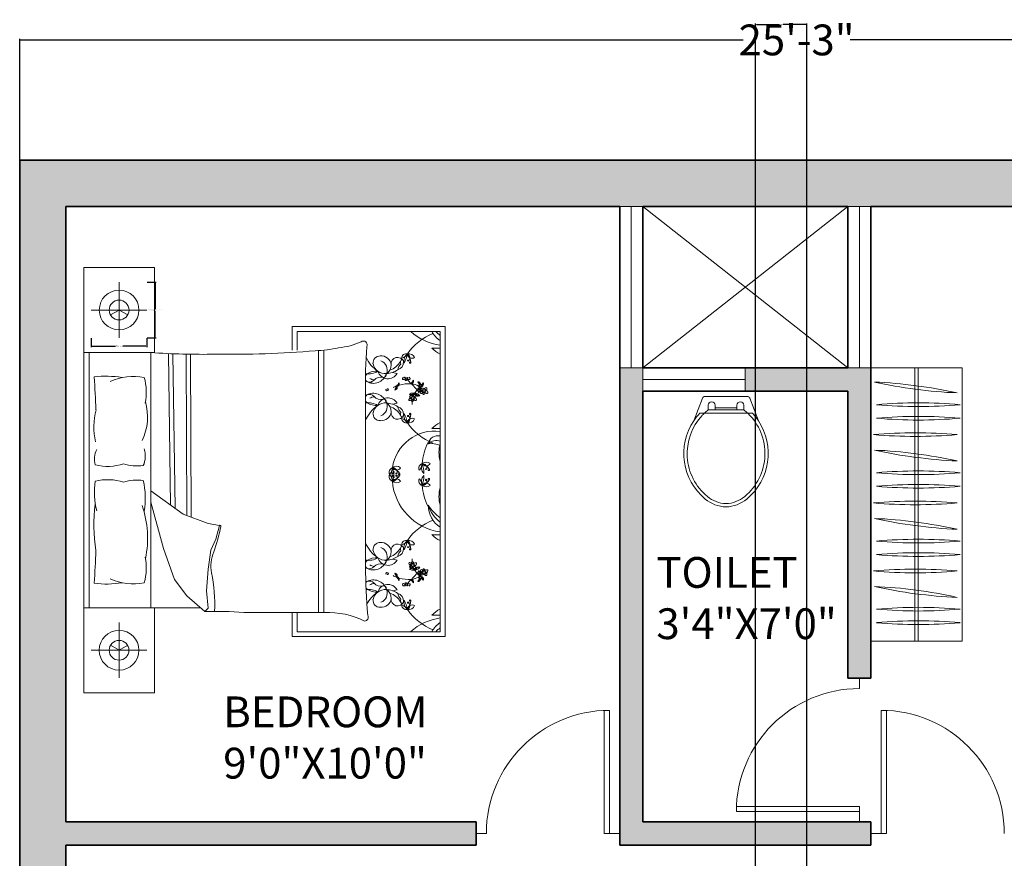
# Model space of a CAD drawing. Units: inches. Extents: x -5 to 366, y -496 to 54.
# Tile 9 of 10: x 22 to 214, y -110 to 54. Entities that reach past the tile are written whole.
import ezdxf

# ---------------------------------------------------------------- set-up
doc = ezdxf.new("R2010")
doc.units = ezdxf.units.IN
doc.header["$MEASUREMENT"] = 0
for name, color, linetype, lineweight in [('A-ANNO-DIMS', 2, 'Continuous', 18), ('A-AREA-IDEN', 7, 'Continuous', 25), ('A-DOOR', 3, 'Continuous', 18), ('A-FLOR-FIXT', 9, 'Continuous', 18), ('A-FLOR-OPEN', 8, 'Continuous', 13), ('A-FURN', 8, 'Continuous', 18), ('A-GLAZ', 4, 'Continuous', 18), ('A-WALL', 7, 'Continuous', 35), ('A-WALL-PATT', 252, 'Continuous', 13)]:
    doc.layers.add(name, color=color, linetype=linetype, lineweight=lineweight)
doc.styles.get("Standard").update_dxf_attribs({"font": 'arial.ttf'})
doc.dimstyles.get("Standard").update_dxf_attribs({"dimtxt": 0.18, "dimasz": 0.18, "dimexe": 0.18, "dimexo": 0.0625, "dimgap": 0.09, "dimtad": 0, "dimtih": 1, "dimtoh": 1, "dimdec": 0, "dimzin": 0, "dimdsep": 46, "dimlunit": 3, "dimtxsty": 'Standard', "dimcen": 0.09, "dimadec": 0, "dimazin": 0, "dimtfac": 1, "dimtdec": 0, "dimtofl": 0, "dimtmove": 0, "dimatfit": 3, "dimfxl": 1, "dimtolj": 1, "dimtzin": 0, "dimarcsym": 0})

# ---------------------------------------------------------------- blocks, each defined once
blk = doc.blocks.new('*D2')
at = {"layer": 'A-ANNO-DIMS', "color": 0, "lineweight": -2, "transparency": 16777216}
for p, q in [((21.93, 26.58), (21.93, 50.16)), ((22.11, 49.98), (162.99, 49.98)), ((324.75, 49.98), (183.88, 49.98)), ((324.93, 26.58), (324.93, 50.16))]:
    blk.add_line(p, q, dxfattribs=at)
at = {"layer": 'A-ANNO-DIMS', "color": 0, "transparency": 16777216}
for points in [[(22.11, 50.01), (22.11, 49.95), (21.93, 49.98)], [(324.75, 50.01), (324.75, 49.95), (324.93, 49.98)]]:
    blk.add_solid(points, dxfattribs=at)
at = {"layer": 'Defpoints', "color": 0, "transparency": 16777216}
for p in [(324.93, 49.98), (21.93, 26.52), (324.93, 26.52)]:
    blk.add_point(p, dxfattribs=at)
at = {"layer": 'A-ANNO-DIMS', "color": 0, "transparency": 16777216, "insert": (173.43, 49.98), "char_height": 6, "attachment_point": 5}
blk.add_mtext('\\A1;25\'-3"', dxfattribs=at)
blk = doc.blocks.new('DOOR-SWING-24IN')
for p, q in [((-1, 0), (-1, 24)), ((0, 0), (0, 24))]:
    blk.add_line(p, q)
blk.add_arc((0, 0), 24, 90, 180)
blk = doc.blocks.new('WARDROBE-HANGING')
for p, q in [((0, 53.26), (0, 0)), ((0, 53.26), (17.76, 53.26)), ((8.58, 53.26), (8.58, 0)), ((9.18, 53.26), (9.18, 0)), ((17.76, 53.26), (17.76, 0)), ((0, 0), (17.76, 0))]:
    blk.add_line(p, q)
for centre, start, end in [((20.87, 141.73), 257.508, 267.5023), ((-3.4, -42.81), 77.508, 87.5023), ((9.24, -46.96), 85.0028, 94.9972), ((9.24, 139.16), 265.0028, 274.9972), ((9.24, -49.59), 85.0028, 94.9972), ((9.24, 136.53), 265.0028, 274.9972), ((8.66, -52.79), 85.0028, 94.9972), ((8.66, 133.34), 265.0028, 274.9972), ((20.87, 128.46), 257.508, 267.5023), ((-3.4, -56.08), 77.508, 87.5023), ((9.24, -60.23), 85.0028, 94.9972), ((9.24, 125.89), 265.0028, 274.9972), ((9.24, -62.86), 85.0028, 94.9972), ((9.24, 123.26), 265.0028, 274.9972), ((8.66, -66.11), 85.0028, 94.9972), ((8.66, 120.02), 265.0028, 274.9972), ((-3.4, -69.4), 77.508, 87.5023), ((20.87, 115.14), 257.508, 267.5023), ((9.24, -73.55), 85.0028, 94.9972), ((9.24, 112.57), 265.0028, 274.9972), ((9.24, -76.18), 85.0028, 94.9972), ((9.24, 109.94), 265.0028, 274.9972), ((8.66, -79.38), 85.0028, 94.9972), ((8.66, 106.75), 265.0028, 274.9972), ((-3.4, -82.67), 77.508, 87.5023), ((20.87, 101.87), 257.508, 267.5023), ((9.24, -86.82), 85.0028, 94.9972), ((9.24, 99.3), 265.0028, 274.9972), ((9.24, -89.45), 85.0028, 94.9972), ((9.24, 96.67), 265.0028, 274.9972)]:
    blk.add_arc(centre, 93.42, start, end)
blk = doc.blocks.new('LAMP-BEDSIDE')
for p, q in [((5.42, 0), (5.42, 10.83)), ((10.83, 5.42), (0, 5.42))]:
    blk.add_line(p, q)
for points in [[(5.42, 5.42), (3.74, 4.45)], [(5.42, 5.42), (7.09, 4.45)]]:
    blk.add_lwpolyline(points)
for radius in [3.87, 1.93]:
    blk.add_circle((5.42, 5.42), radius)
blk = doc.blocks.new('*D23')
at = {"layer": 'A-ANNO-DIMS', "color": 0, "lineweight": -2, "transparency": 16777216}
for p, q in [((46.8, 2.73), (48.54, 2.73)), ((48.36, 2.55), (48.36, -2.5)), ((48.36, -7.92), (48.36, -2.87)), ((46.8, -8.1), (48.54, -8.1))]:
    blk.add_line(p, q, dxfattribs=at)
at = {"layer": 'A-ANNO-DIMS', "color": 0, "transparency": 16777216}
for points in [[(48.33, 2.55), (48.39, 2.55), (48.36, 2.73)], [(48.33, -7.92), (48.39, -7.92), (48.36, -8.1)]]:
    blk.add_solid(points, dxfattribs=at)
at = {"layer": 'Defpoints', "color": 0, "transparency": 16777216}
for p in [(46.73, 2.73), (48.36, 2.73), (46.73, -8.1)]:
    blk.add_point(p, dxfattribs=at)
at = {"layer": 'A-ANNO-DIMS', "color": 0, "transparency": 16777216, "insert": (48.36, -2.68), "char_height": 0.18, "attachment_point": 5}
blk.add_mtext('\\A1;BEDSIDE LAMP 0\'-11" TYP.', dxfattribs=at)
blk = doc.blocks.new('*D24')
at = {"layer": 'A-ANNO-DIMS', "color": 0, "lineweight": -2, "transparency": 16777216}
for p, q in [((35.9, -8.16), (35.9, -9.9)), ((46.73, -8.16), (46.73, -9.9)), ((36.08, -9.72), (40.61, -9.72)), ((46.55, -9.72), (42.02, -9.72))]:
    blk.add_line(p, q, dxfattribs=at)
at = {"layer": 'A-ANNO-DIMS', "color": 0, "transparency": 16777216}
for points in [[(36.08, -9.69), (36.08, -9.75), (35.9, -9.72)], [(46.55, -9.69), (46.55, -9.75), (46.73, -9.72)]]:
    blk.add_solid(points, dxfattribs=at)
at = {"layer": 'Defpoints', "color": 0, "transparency": 16777216}
for p in [(35.9, -8.1), (46.73, -8.1), (46.73, -9.72)]:
    blk.add_point(p, dxfattribs=at)
at = {"layer": 'A-ANNO-DIMS', "color": 0, "transparency": 16777216, "insert": (41.32, -9.72), "char_height": 0.18, "attachment_point": 5}
blk.add_mtext('\\A1;0\'-11" TYP.', dxfattribs=at)
blk = doc.blocks.new('*D29')
at = {"layer": 'A-ANNO-DIMS', "color": 0, "lineweight": -2, "transparency": 16777216}
for p, q in [((165.43, -380.42), (165.43, 53.15)), ((165.61, 52.97), (170.03, 52.97)), ((175.25, 52.97), (170.83, 52.97)), ((175.43, -380.42), (175.43, 53.15))]:
    blk.add_line(p, q, dxfattribs=at)
at = {"layer": 'A-ANNO-DIMS', "color": 0, "transparency": 16777216}
for points in [[(165.61, 53), (165.61, 52.94), (165.43, 52.97)], [(175.25, 53), (175.25, 52.94), (175.43, 52.97)]]:
    blk.add_solid(points, dxfattribs=at)
at = {"layer": 'Defpoints', "color": 0, "transparency": 16777216}
for p in [(175.43, 52.97), (165.43, -380.48), (175.43, -380.48)]:
    blk.add_point(p, dxfattribs=at)
at = {"layer": 'A-ANNO-DIMS', "color": 0, "transparency": 16777216, "insert": (170.43, 52.97), "char_height": 0.18, "attachment_point": 5}
blk.add_mtext('\\A1;0\'-10"', dxfattribs=at)

msp = doc.modelspace()

# ---------------------------------------------------------------- hatches: boundary and pattern name
at = {"layer": 'A-WALL-PATT'}
h = msp.add_hatch(color=256, dxfattribs=at)
h.dxf.hatch_style = 1
h.paths.add_polyline_path([(324.93, 26.52), (21.93, 26.52), (21.93, -456.98), (26.43, -456.98), (26.43, -331.98), (30.93, -331.98), (30.93, -322.98), (30.93, -106.98), (110.93, -106.98), (110.93, -104.73), (110.93, -102.48), (30.93, -102.48), (30.93, 17.52), (138.93, 17.52), (141.18, 17.52), (143.43, 17.52), (183.43, 17.52), (187.93, 17.52), (315.93, 17.52), (315.93, -102.48), (315.93, -106.98), (315.93, -255.48), (171.93, -255.48), (171.93, -155.84), (167.43, -155.84), (167.43, -291.98), (171.93, -291.98), (171.93, -259.98), (315.93, -259.98), (315.93, -375.98), (297.93, -375.98), (297.93, -380.48), (315.93, -380.48), (315.93, -452.48), (315.93, -456.98), (324.93, -456.98)])
h.paths.add_polyline_path([(143.43, -18.48), (143.43, -13.98), (138.93, -13.98), (138.93, -106.98), (187.93, -106.98), (187.93, -102.48), (143.43, -102.48)], flags=17)
h = msp.add_hatch(color=256, dxfattribs=at)
h.dxf.hatch_style = 1
h.paths.add_polyline_path([(187.93, -13.98), (183.43, -13.98), (163.43, -13.98), (163.43, -18.48), (183.43, -18.48), (183.43, -74.48), (185.68, -74.48), (187.93, -74.48)])
h.paths.add_polyline_path([(284.93, -102.48), (215.93, -102.48), (215.93, -104.73), (215.93, -106.98), (280.43, -106.98), (284.93, -106.98)])
h.paths.add_polyline_path([(284.93, -133.23), (280.43, -133.23), (280.43, -154.98), (220.43, -154.98), (220.43, -134.98), (215.93, -134.98), (215.93, -159.48), (284.93, -159.48)])
h.paths.add_polyline_path([(139.43, -322.98), (123.64, -322.98), (123.64, -331.98), (139.43, -331.98)])
h.paths.add_polyline_path([(171.93, -319.98), (167.43, -319.98), (167.43, -331.98), (171.93, -331.98)])
h.paths.add_polyline_path([(269.93, -375.98), (171.93, -375.98), (167.43, -375.98), (167.43, -380.48), (171.93, -380.48), (265.43, -380.48), (265.43, -452.48), (171.93, -452.48), (167.43, -452.48), (167.43, -456.98), (281.67, -456.98), (281.67, -452.48), (269.93, -452.48), (269.93, -380.48)])

# ---------------------------------------------------------------- linework, layer by layer
at = {"layer": 'A-DOOR'}
for p, q in [((185.68, -76.48), (185.68, -74.48)), ((185.68, -102.48), (185.68, -99.48)), ((112.93, -104.73), (110.93, -104.73)), ((138.93, -104.73), (135.93, -104.73)), ((187.93, -104.73), (190.93, -104.73))]:
    msp.add_line(p, q, dxfattribs=at)
at = {"layer": 'A-FLOR-FIXT'}
for p, q in [((154.53, -22.8), (155.43, -22.8)), ((155.43, -22.8), (159.67, -22.8)), ((163.91, -22.8), (159.67, -22.8)), ((163.91, -22.8), (164.81, -22.8))]:
    msp.add_line(p, q, dxfattribs=at)
for points in [[(159.67, -19.54), (155.56, -19.54, 0.31031), (155.05, -19.89), (153.36, -24.28, 0.209071)], [(156.18, -22.15), (156.18, -21.25, -1), (157.55, -21.25), (157.55, -21.72)], [(159.67, -19.54), (163.78, -19.54, -0.31031), (164.29, -19.89), (165.98, -24.28, -0.209071)], [(163.16, -22.15), (163.16, -21.25, 1), (161.79, -21.25), (161.79, -21.72)], [(154.53, -22.8, 0.040937), (153.36, -24.28, 0.163732)], [(155.43, -22.8, 0.014165), (155, -23.24, 0.162618)], [(156.18, -22.15, 0.022712), (155.43, -22.8, 0.162618)], [(159.67, -22.15), (156.18, -22.15, 0.022712)], [(159.67, -22.15), (163.16, -22.15, -0.476108)], [(163.91, -22.8, -0.448546), (163.31, -39.03, -0.162618), (159.67, -40.43, -0.470877)], [(163.16, -22.15, -0.022712), (163.91, -22.8, -0.162618)], [(164.81, -22.8, -0.040937), (165.98, -24.28, -0.163732)], [(153.36, -24.28, 0.383919), (155.62, -39.53, 0.163732), (159.67, -41.08, 0.359733)], [(155, -23.24, 0.431639), (156.03, -39.03, 0.162618), (159.67, -40.43, 0.470877)], [(165.98, -24.28, -0.383919), (163.72, -39.53, -0.163732), (159.67, -41.08, -0.359733)]]:
    msp.add_lwpolyline(points, format="xyb", dxfattribs=at)
for points in [[(161.79, -21.72), (157.55, -21.72)], [(157.55, -21.72), (157.55, -22.15)], [(161.79, -21.72), (161.79, -22.15)]]:
    msp.add_lwpolyline(points, dxfattribs=at)
at = {"layer": 'A-FLOR-OPEN'}
for p, q in [((143.43, 17.52), (183.43, -13.98)), ((183.43, 17.52), (143.43, -13.98))]:
    msp.add_line(p, q, dxfattribs=at)
at = {"layer": 'A-FURN'}
for p, q in [((34.41, -77.29), (34.41, 5.61)), ((75.05, -10.51), (75.05, -5.91)), ((75.05, -5.91), (104.91, -5.91)), ((76.01, -6.87), (76.01, -10.53)), ((103.95, -6.87), (76.01, -6.87)), ((103.95, -65.39), (103.95, -6.87)), ((104.91, -5.91), (104.91, -66.35)), ((35.47, -10.97), (35.47, -60.71)), ((47.51, -60.71), (47.51, -10.97)), ((50.95, -11.2), (51.37, -40.71)), ((51.8, -11.23), (52.23, -41.33)), ((54.41, -11.27), (54.54, -42.75)), ((55.26, -11.27), (55.4, -43.08)), ((80.22, -10.6), (80.22, -61.67)), ((81.25, -10.52), (81.25, -61.67)), ((95.54, -15.04), (94.61, -14.86)), ((89.39, -19.01), (89.39, -52.67)), ((95.54, -20.84), (94.61, -21.02)), ((47.51, -37.94), (53.83, -42.48)), ((49.97, -49.2), (47.51, -40.16)), ((53.83, -42.48), (58.7, -44.33)), ((58.7, -44.33), (60.88, -44.67)), ((60.88, -44.67), (60.21, -47.35)), ((60.21, -47.35), (59.2, -49.53)), ((52.15, -55.24), (49.97, -49.2)), ((59.2, -49.53), (58.7, -53.23)), ((95.54, -51.43), (94.61, -51.25)), ((58.7, -53.23), (58.36, -57.43)), ((54.5, -58.43), (52.15, -55.24)), ((58.36, -57.43), (58.7, -60.78)), ((95.54, -57.22), (94.61, -57.41)), ((58.03, -61.46), (54.5, -58.43)), ((34.41, -60.71), (57.16, -60.71)), ((58.7, -60.78), (58.03, -61.46)), ((75.05, -66.35), (75.05, -61.66)), ((76.01, -61.67), (76.01, -65.39)), ((104.91, -66.35), (75.05, -66.35)), ((76.01, -65.39), (103.95, -65.39))]:
    msp.add_line(p, q, dxfattribs=at)
for points in [[(34.41, -10.97), (48.22, -10.97), (48.22, 5.61), (34.41, 5.61)], [(48.22, -60.71), (48.22, -77.29), (34.41, -77.29)]]:
    msp.add_lwpolyline(points, dxfattribs=at)
for points in [[(79.56, -10.62, 0.056112), (84.13, -10.02, 0.095341), (88.52, -8.85)], [(36.47, -15.73, -0.074897), (41.89, -15.84, 0.472817)], [(42.19, -32.69, -0.14099), (36.67, -32.86, -0.235245)], [(42.19, -36.23, 0.14099), (36.67, -36.07, 0.235245)], [(36.47, -55.95, 0.074897), (41.89, -55.85, -0.472817)], [(65.62, -61.63, 0.001242), (81.35, -61.67, -0.127202), (89.19, -63.33)]]:
    msp.add_lwpolyline(points, format="xyb", dxfattribs=at)
for centre in [(100.77, -18.45), (98.55, -19.83), (98.55, -52.43), (100.77, -53.81)]:
    msp.add_circle(centre, 0.211, dxfattribs=at)
for centre, radius, start, end in [((106.48, -17.34), 10.83, 111.4092, 145.6135), ((105.41, 1.19), 10.83, 228.1144, 262.255), ((106.86, -4.25), 5.28, 209.8884, 236.5383), ((107.84, -2.35), 6.57, 223.5186, 233.6964), ((88.94, -9.48), 0.756, 336.5219, 123.8264), ((57.64, 137.64), 148.96, 266.1, 270.9282), ((63.06, 182.99), 194.31, 269.1145, 274.8735), ((170.02, -16.48), 80.67, 175.2402, 181.8035), ((97.33, -12.09), 0.897, 76.272, 177.0484), ((95.97, -10.26), 1.85, 284.7031, 328.6173), ((98.55, -12.61), 1.71, 125.7657, 194.5347), ((90.15, -9.58), 7.57, 332.8176, 347.4827), ((97.8, -12.39), 1.2, 20.9613, 102.2885), ((98.45, -11.19), 0.904, 181.7131, 301.5367), ((95.48, -13.02), 2.74, 2.0648, 41.1598), ((97.13, -12.01), 0.886, 316.2238, 62.3173), ((105.64, -7.2), 4.4, 221.0454, 247.4453), ((103.27, 4.86), 14.98, 266.3481, 272.5919), ((95.23, -9.37), 6.27, 203.6453, 236.3329), ((92.22, -13.03), 1.4, 88.9462, 185.5144), ((93.26, -12.6), 2.49, 193.079, 274.7067), ((92.42, -13.6), 1.98, 7.1143, 95.0551), ((91.67, -14.38), 1.92, 338.5779, 68.4181), ((91.98, -13.26), 2.41, 305.9599, 357.6409), ((92.87, -10.68), 3.91, 288.2955, 328.7386), ((95.61, -13.15), 1.24, 19.1312, 189.736), ((95.24, -12.85), 1.55, 285.6955, 4.031), ((97.3, -14.52), 1.65, 128.4175, 173.8338), ((96.96, -12.89), 0.763, 126.7319, 206.0245), ((97.64, -12.52), 0.0706, 20.2667, 316.2271), ((98.02, -12.92), 0.0653, 52.0591, 168.5166), ((98.09, -12.93), 0.134, 168.5166, 2.0648), ((90.31, -15.93), 0.998, 127.675, 162.5814), ((90.01, -11.68), 3.43, 259.249, 301.1782), ((90.9, -14.34), 2.64, 240.8249, 340.7178), ((91.5, -17.78), 3.2, 85.2696, 124.215), ((93.76, -14.02), 2.06, 196.8663, 330.0915), ((92.89, -15.32), 0.515, 254.8529, 12.6959), ((91.5, -17.78), 3.2, 53.6555, 57.2989), ((93.19, -10.64), 4.45, 273.4924, 303.7117), ((-752.48, -61.43), 790.27, 2.85022, 3.31479), ((44.06, -26.3), 10.68, 78.2417, 114.8684), ((35.5, -18.69), 11.11, 348.9631, 14.8961), ((90.31, -15.93), 0.998, 196.6343, 225.5483), ((90.11, -15.51), 1.24, 246.1646, 318.4347), ((91.38, -13.94), 2.38, 240.0851, 262.564), ((92.31, -17.46), 1.7, 74.8529, 138.4347), ((95.54, -17.17), 0.398, 265.7131, 351.6568), ((94.67, -16.35), 1.33, 313.6929, 321.7899), ((96.14, -17.26), 0.435, 115.5379, 168.6744), ((94.67, -16.64), 1.31, 329.344, 349.7412), ((97.85, -23.93), 6.87, 86.1723, 106.4158), ((93.62, -16.94), 2.34, 352.8698, 1.6736), ((96.72, -16.1), 0.163, 125.0752, 284.7644), ((96.97, -16.03), 0.352, 127.3642, 168.4363), ((96.69, -15.75), 0.508, 277.4968, 341.2737), ((97.09, -15.99), 0.202, 88.1325, 178.8919), ((97.5, -16.2), 0.436, 136.3462, 189.6513), ((97.25, -16.24), 0.182, 189.6513, 312.3208), ((97.29, -15.74), 0.211, 183.2768, 356.7232), ((97.95, -16.12), 0.691, 164.2829, 186.9148), ((97.14, -16.12), 0.345, 312.3208, 40.2111), ((97.87, -15.73), 0.491, 201.6382, 274.947), ((97.22, -16.4), 0.641, 42.3896, 66.5724), ((103.69, -11.33), 7.87, 217.9541, 226.8459), ((97.68, -16.03), 0.349, 10.9597, 52.2379), ((97.9, -16.06), 0.162, 274.947, 37.5263), ((98.44, -16.98), 0.169, 112.5583, 214.2343), ((98.33, -16.68), 0.398, 265.7131, 351.6568), ((97.98, -16.46), 0.695, 297.3659, 329.344), ((98.02, -20.5), 3.44, 60.7959, 85.244), ((90.69, -25.46), 11.33, 37.8256, 47.7588), ((97.46, -15.86), 1.33, 313.6929, 321.7899), ((98.93, -16.77), 0.435, 115.5379, 168.6744), ((97.45, -16.14), 1.31, 329.344, 349.7412), ((96.41, -16.44), 2.34, 352.8698, 1.6736), ((99.7, -16.92), 0.236, 33.0979, 123.1364), ((94.5, -20.24), 6.17, 31.1156, 34.8118), ((99.35, -17.32), 0.638, 2.3172, 70.5201), ((99.57, -17.18), 0.244, 315.7354, 31.1156), ((99.59, -17.25), 0.55, 352.6008, 57.1845), ((100.12, -17.13), 0.55, 252.8042, 349.6943), ((100.18, -17.08), 0.244, 248.2452, 323.6254), ((99.96, -16.93), 0.638, 291.7087, 3.0299), ((95.41, -13.57), 6.17, 323.6254, 327.3216), ((100.47, -17.09), 0.236, 325.6077, 55.6462), ((90.9, -21.55), 2.64, 19.2822, 119.1751), ((90.11, -20.37), 1.24, 41.5653, 113.8354), ((93.57, -18.16), 0.26, 169.5864, 349.5616), ((93.67, -18.18), 0.16, 349.5616, 167.2949), ((97.85, -23.93), 6.87, 110.1059, 116.9968), ((95.54, -18.27), 0.435, 129.5056, 182.6421), ((94.29, -17.26), 1.31, 308.4388, 328.836), ((94.06, -16.19), 2.34, 296.5064, 305.3102), ((94.04, -17.4), 1.33, 336.3901, 344.4871), ((95.5, -17.74), 0.169, 83.9457, 185.6216), ((94.82, -17.58), 0.695, 328.836, 0.8141), ((95.18, -17.78), 0.398, 306.5232, 32.4668), ((95.65, -17.47), 0.169, 112.5583, 214.2343), ((95.19, -16.95), 0.695, 297.3659, 329.344), ((98.23, -18.22), 0.962, 253.6301, 325.4631), ((98.51, -19.55), 0.681, 82.0748, 142.6895), ((98.43, -18.62), 0.699, 228.342, 274.9894), ((98.45, -18.73), 0.585, 273.8774, 357.1501), ((98.68, -18.32), 0.566, 262.0748, 308.2393), ((102.59, -20.86), 4.13, 156.1523, 156.9499), ((98.95, -19.39), 0.209, 44.3732, 121.9501), ((99.59, -18.9), 0.585, 181.4625, 249.4747), ((102.59, -20.86), 4.13, 130.182, 149.456), ((99.49, -18.44), 0.566, 215.1128, 261.2773), ((99.94, -18.47), 0.962, 197.889, 269.722), ((99.3, -19.67), 0.681, 20.6625, 81.2773), ((100.32, -18.51), 0.681, 139.3812, 199.9959), ((99.05, -18.01), 0.962, 310.9365, 22.7695), ((99.49, -18.07), 0.699, 285.6484, 332.2957), ((99.88, -17.48), 0.184, 135.7354, 318.1297), ((99.37, -17.69), 0.566, 319.3812, 5.5456), ((100.02, -17.48), 0.184, 68.2452, 250.6395), ((101.56, -20.94), 3.68, 111.7087, 116.2181), ((98.02, -20.5), 3.44, 47.5083, 55.9967), ((99.59, -18.11), 0.585, 331.1838, 51.6792), ((100.2, -18.81), 0.163, 125.0752, 284.7644), ((100.45, -18.74), 0.352, 93.635, 168.4363), ((100.4, -18.19), 0.207, 138.2946, 276.2474), ((100.17, -18.46), 0.508, 277.4968, 341.2737), ((100.48, -18.22), 0.288, 358.5719, 143.8954), ((100.57, -18.7), 0.202, 88.1325, 178.8919), ((100.65, -17.99), 0.291, 208.8493, 269.9355), ((100.4, -18.06), 0.332, 274.2123, 318.1587), ((100.98, -18.91), 0.436, 136.3462, 189.6513), ((100.73, -18.96), 0.182, 189.6513, 312.3208), ((101.43, -18.83), 0.691, 164.2829, 186.9148), ((101.41, -18.4), 0.666, 121.9501, 165.2442), ((100.62, -18.83), 0.345, 312.3208, 40.2111), ((101.35, -18.45), 0.491, 201.6382, 274.947), ((100.95, -18.14), 0.14, 262.868, 7.094), ((100.7, -19.12), 0.641, 42.3896, 66.5724), ((100.94, -18.02), 0.417, 278.5614, 22.5914), ((101.17, -18.74), 0.349, 10.9597, 118.7804), ((101.17, -18.01), 0.209, 44.3732, 121.9501), ((101.38, -18.77), 0.162, 274.947, 37.5263), ((36.32, -23.49), 10.55, 333.8761, 16.1746), ((90.31, -19.95), 0.998, 134.4517, 156.7144), ((90.31, -19.95), 0.998, 203.2856, 232.325), ((90.01, -24.21), 3.43, 58.8218, 100.2867), ((91.5, -18.1), 3.2, 235.785, 274.7304), ((91.38, -21.94), 2.38, 97.436, 119.9149), ((93.26, -23.28), 2.49, 85.2933, 166.921), ((92.31, -18.42), 1.7, 221.5653, 285.1471), ((93.76, -21.87), 2.06, 29.9085, 163.1337), ((91.67, -21.5), 1.92, 291.5819, 21.4221), ((92.89, -20.56), 0.515, 347.3041, 105.1471), ((91.5, -18.1), 3.2, 302.7011, 306.3445), ((91.98, -22.62), 2.41, 2.3591, 54.0401), ((93.19, -25.24), 4.45, 56.2883, 86.5076), ((97.97, -20.19), 0.163, 125.0752, 284.7644), ((98.22, -20.13), 0.352, 93.635, 168.4363), ((98.18, -19.57), 0.207, 138.2946, 276.2474), ((97.95, -19.84), 0.508, 277.4968, 341.2737), ((98.26, -19.6), 0.288, 358.5719, 143.8954), ((98.35, -20.08), 0.202, 88.1325, 178.8919), ((98.42, -19.37), 0.291, 208.8493, 269.9355), ((98.18, -19.44), 0.332, 274.2123, 318.1587), ((98.75, -20.29), 0.436, 136.3462, 189.6513), ((98.5, -20.34), 0.182, 189.6513, 312.3208), ((102.59, -20.86), 4.13, 175.2415, 182.8929), ((99.21, -20.21), 0.691, 164.2829, 186.9148), ((99.19, -19.78), 0.666, 121.9501, 165.2442), ((98.39, -20.22), 0.345, 312.3208, 40.2111), ((99.13, -19.83), 0.491, 201.6382, 274.947), ((98.73, -19.52), 0.14, 262.868, 7.094), ((98.48, -20.5), 0.641, 42.3896, 66.5724), ((98.71, -19.4), 0.417, 278.5614, 22.5914), ((98.94, -20.12), 0.349, 10.9597, 118.7804), ((99.15, -20.15), 0.162, 274.947, 37.5263), ((99.64, -18.8), 0.699, 248.3627, 295.0101), ((50.98, -25.57), 14.57, 166.3427, 191.1841), ((95.23, -26.51), 6.27, 123.6671, 158.5059), ((92.22, -22.85), 1.4, 174.4856, 271.0538), ((92.42, -22.28), 1.98, 264.9449, 352.8857), ((92.87, -25.2), 3.91, 31.2614, 71.7045), ((95.61, -22.73), 1.24, 170.264, 340.8688), ((97.3, -21.36), 1.65, 186.1662, 231.5825), ((95.24, -23.03), 1.55, 355.969, 74.3045), ((96.96, -22.99), 0.763, 153.9755, 233.2681), ((98.55, -23.27), 1.71, 165.4653, 234.2343), ((90.15, -26.3), 7.57, 12.5173, 27.1824), ((95.48, -22.86), 2.74, 318.8402, 357.9352), ((98.09, -22.95), 0.134, 357.9352, 191.4834), ((98.02, -22.97), 0.0653, 191.4834, 307.9409), ((97.33, -23.79), 0.897, 182.9516, 283.728), ((95.97, -25.62), 1.85, 31.3827, 75.2969), ((97.13, -23.88), 0.886, 297.6827, 43.7762), ((98.45, -24.69), 0.904, 58.4633, 178.2869), ((97.8, -23.49), 1.2, 257.7115, 339.0387), ((106.48, -18.55), 10.83, 214.3865, 248.5908), ((97.69, -23.34), 0.117, 43.7762, 339.7183), ((105.64, -28.68), 4.4, 112.5547, 138.9546), ((102.91, -34.65), 8.38, 82.8636, 171.8197), ((103.27, -40.74), 14.98, 87.4081, 93.6519), ((111.21, -33.47), 10.83, 152.5854, 175.5377), ((103.49, -29.12), 1.94, 76.3898, 169.0739), ((103.23, -30.58), 2.46, 72.8609, 131.9049), ((102.14, -33.57), 4.85, 68.117, 96.6195), ((109.64, -30.45), 5.95, 162.9798, 196.4569), ((40.61, -31.72), 4.1, 153.3437, 196.1026), ((42.04, -31.17), 4.39, 335.0183, 18.5407), ((100.66, -33.49), 0.897, 106.1963, 206.9726), ((98.57, -32.59), 1.85, 314.6273, 358.5415), ((101.97, -33.34), 1.71, 155.6899, 224.4589), ((101.22, -33.52), 1.2, 50.8855, 132.2127), ((101.18, -32.16), 0.904, 211.6373, 331.4609), ((99.53, -35.22), 2.74, 31.989, 71.0841), ((93.19, -34.9), 7.57, 2.7418, 17.407), ((100.45, -33.52), 0.886, 346.148, 92.2415), ((112.71, -32.81), 8.8, 174.3643, 175.6213), ((118.74, -37.44), 15.73, 160.0972, 160.2783), ((44.96, -22.92), 10.16, 254.1707, 275.9871), ((94.87, -34.32), 0.897, 106.1963, 206.9726), ((92.77, -33.41), 1.85, 314.6273, 358.5415), ((96.18, -34.17), 1.71, 155.6899, 224.4589), ((96.18, -35.34), 1.71, 135.5411, 204.3101), ((95.42, -34.35), 1.2, 50.8855, 132.2127), ((95.39, -32.99), 0.904, 211.6373, 331.4609), ((94.65, -34.35), 0.886, 346.148, 92.2415), ((93.73, -36.05), 2.74, 31.989, 71.0841), ((87.39, -35.73), 7.57, 2.7418, 17.407), ((87.39, -33.78), 7.57, 342.593, 357.2582), ((95.35, -34.54), 0.0706, 50.1909, 346.0209), ((101.15, -33.71), 0.0706, 50.1909, 346.0209), ((101.67, -33.87), 0.0653, 81.9833, 198.4408), ((101.73, -33.84), 0.134, 198.4408, 31.989), ((51.28, -38.24), 14.77, 171.5249, 193.96), ((44.96, -46), 10.16, 84.0129, 105.8293), ((31.81, -39.35), 14.62, 349.8617, 13.6238), ((94.87, -35.18), 0.897, 153.0274, 253.8037), ((92.77, -36.09), 1.85, 1.4585, 45.3727), ((93.73, -33.45), 2.74, 288.9159, 328.011), ((94.65, -35.16), 0.886, 267.7585, 13.852), ((95.39, -36.52), 0.904, 28.5391, 148.3627), ((95.42, -35.15), 1.2, 227.7873, 309.1145), ((105.41, -35.2), 10.83, 184.4623, 262.255), ((95.4, -34.97), 0.117, 13.852, 309.9245), ((95.94, -34.67), 0.134, 198.4408, 31.989), ((95.87, -34.69), 0.0653, 81.9833, 198.4408), ((95.94, -34.83), 0.134, 328.011, 161.5592), ((95.87, -34.81), 0.0653, 161.5592, 278.0167), ((100.66, -36.01), 0.897, 153.0274, 253.8037), ((98.57, -36.92), 1.85, 1.4585, 45.3727), ((101.97, -36.17), 1.71, 135.5411, 204.3101), ((93.19, -34.6), 7.57, 342.593, 357.2582), ((99.53, -34.28), 2.74, 288.9159, 328.011), ((100.45, -35.99), 0.886, 267.7585, 13.852), ((101.18, -37.34), 0.904, 28.5391, 148.3627), ((101.19, -35.8), 0.117, 13.852, 309.9245), ((101.67, -35.64), 0.0653, 161.5592, 278.0167), ((101.73, -35.66), 0.134, 328.011, 161.5592), ((101.22, -35.98), 1.2, 227.7873, 309.1145), ((111.21, -36.03), 10.83, 184.4623, 207.4146), ((109.64, -39.06), 5.95, 163.5431, 197.0202), ((112.71, -36.7), 8.8, 184.3787, 185.6357), ((118.74, -32.06), 15.73, 199.7217, 199.9028), ((66.47, -44.59), 30.07, 172.2196, 189.497), ((27.61, -47.15), 19.27, 348.0397, 19.2615), ((106.86, -40.63), 5.28, 181.272, 236.5383), ((109.69, -35.28), 9.78, 214.0123, 234.053), ((107.84, -38.73), 6.57, 197.8504, 233.6964), ((106.48, -53.72), 10.83, 111.4092, 145.6135), ((29.55, -38.91), 32.15, 340.1194, 349.3383), ((60.95, -44.85), 0.2, 358.8623, 109.7536), ((97.33, -48.48), 0.897, 76.272, 177.0484), ((95.97, -46.64), 1.85, 284.7031, 328.6173), ((98.55, -49), 1.71, 125.7657, 194.5347), ((90.15, -45.97), 7.57, 332.8176, 347.4827), ((97.8, -48.78), 1.2, 20.9613, 102.2885), ((97.13, -48.39), 0.886, 316.2238, 62.3173), ((95.48, -49.41), 2.74, 2.0648, 41.1598), ((98.45, -47.58), 0.904, 181.7131, 301.5367), ((103.27, -31.53), 14.98, 266.3481, 272.5919), ((105.64, -43.58), 4.4, 221.0454, 247.4453), ((-752.48, -10.26), 790.27, 356.68521, 357.14978), ((65.96, -52.56), 6.75, 156.2616, 191.3392), ((95.23, -45.76), 6.27, 201.4941, 236.3329), ((92.22, -49.41), 1.4, 88.9462, 185.5144), ((93.26, -48.98), 2.49, 193.079, 274.7067), ((92.42, -49.99), 1.98, 7.1143, 95.0551), ((91.67, -50.77), 1.92, 338.5779, 68.4181), ((91.98, -49.64), 2.41, 305.9599, 357.6409), ((92.87, -47.07), 3.91, 288.2955, 328.7386), ((95.61, -49.53), 1.24, 19.1312, 189.736), ((95.24, -49.23), 1.55, 285.6955, 4.031), ((97.3, -50.91), 1.65, 128.4175, 173.8338), ((96.96, -49.28), 0.763, 126.7319, 206.0245), ((97.64, -48.91), 0.0706, 20.2667, 316.2271), ((98.02, -49.3), 0.0653, 52.0591, 168.5166), ((98.09, -49.31), 0.134, 168.5166, 2.0648), ((35.5, -53), 11.11, 345.1039, 11.0369), ((90.01, -48.06), 3.43, 259.7133, 301.1782), ((90.31, -52.31), 0.998, 127.675, 156.7144), ((90.9, -50.72), 2.64, 240.8249, 340.7178), ((91.5, -54.17), 3.2, 85.2696, 124.215), ((93.76, -50.4), 2.06, 196.8663, 330.0915), ((92.89, -51.71), 0.515, 254.8529, 12.6959), ((91.5, -54.17), 3.2, 53.6555, 57.2989), ((93.19, -47.03), 4.45, 273.4924, 303.7117), ((98.5, -51.93), 0.182, 47.6792, 170.3487), ((102.59, -51.41), 4.13, 177.1071, 184.7585), ((98.39, -52.05), 0.345, 319.7889, 47.6792), ((175.69, -53.66), 86.3, 179.3433, 185.6887), ((90.31, -52.31), 0.998, 203.229, 225.5483), ((90.11, -51.89), 1.24, 246.1646, 318.4347), ((91.38, -50.32), 2.38, 240.0851, 262.564), ((92.31, -53.84), 1.7, 74.8529, 138.4347), ((97.97, -52.08), 0.163, 75.2356, 234.9248), ((98.22, -52.14), 0.352, 191.5637, 266.365), ((98.43, -53.65), 0.699, 85.0106, 131.658), ((98.23, -54.05), 0.962, 34.5369, 106.3699), ((98.51, -52.71), 0.681, 217.3105, 277.9252), ((98.18, -52.7), 0.207, 83.7526, 221.7054), ((97.95, -52.42), 0.508, 18.7263, 82.5032), ((98.26, -52.67), 0.288, 216.1046, 1.4281), ((98.35, -52.19), 0.202, 181.1081, 271.8675), ((98.42, -52.89), 0.291, 90.0645, 151.1507), ((98.18, -52.82), 0.332, 41.8413, 85.7877), ((90.69, -46.81), 11.33, 312.2412, 322.1744), ((98.75, -51.97), 0.436, 170.3487, 223.6538), ((98.45, -53.54), 0.585, 2.8499, 86.1226), ((99.21, -52.06), 0.691, 173.0852, 195.7171), ((99.19, -52.49), 0.666, 194.7558, 238.0499), ((98.68, -53.95), 0.566, 51.7607, 97.9252), ((99.13, -52.44), 0.491, 85.053, 158.3618), ((98.73, -52.75), 0.14, 352.906, 97.132), ((98.48, -51.77), 0.641, 293.4276, 317.6104), ((98.94, -52.15), 0.349, 241.2196, 349.0403), ((98.71, -52.86), 0.417, 337.4086, 81.4386), ((102.59, -51.41), 4.13, 203.0501, 203.8477), ((98.95, -52.88), 0.209, 238.0499, 315.6268), ((99.59, -53.37), 0.585, 110.5253, 178.5375), ((99.94, -53.8), 0.962, 90.278, 162.111), ((99.49, -53.83), 0.566, 98.7227, 144.8872), ((102.59, -51.41), 4.13, 210.544, 229.818), ((99.15, -52.11), 0.162, 322.4737, 85.053), ((99.64, -53.47), 0.699, 64.9899, 111.6373), ((99.3, -52.6), 0.681, 278.7227, 339.3375), ((100.32, -53.76), 0.681, 160.0041, 220.6188), ((99.05, -54.25), 0.962, 337.2305, 49.0635), ((99.49, -54.2), 0.699, 27.7043, 74.3516), ((100.2, -53.46), 0.163, 75.2356, 234.9248), ((100.45, -53.52), 0.352, 191.5637, 266.365), ((100.17, -53.8), 0.508, 18.7263, 82.5032), ((100.57, -53.57), 0.202, 181.1081, 271.8675), ((100.98, -53.35), 0.436, 170.3487, 223.6538), ((100.73, -53.31), 0.182, 47.6792, 170.3487), ((101.43, -53.44), 0.691, 173.0852, 195.7171), ((100.62, -53.43), 0.345, 319.7889, 47.6792), ((101.35, -53.82), 0.491, 85.053, 158.3618), ((100.7, -53.15), 0.641, 293.4276, 317.6104), ((101.17, -53.53), 0.349, 241.2196, 349.0403), ((101.38, -53.49), 0.162, 322.4737, 85.053), ((44.06, -45.39), 10.68, 245.1316, 281.7583), ((28.67, -60.04), 31.29, 357.4519, 11.3392), ((90.31, -56.34), 0.998, 134.4517, 153.558), ((90.9, -57.93), 2.64, 19.2822, 119.1751), ((90.11, -56.76), 1.24, 41.5653, 113.8354), ((93.57, -54.11), 0.26, 10.4384, 190.4136), ((93.67, -54.09), 0.16, 192.7051, 10.4384), ((97.85, -48.34), 6.87, 243.0032, 249.8941), ((94.29, -55.01), 1.31, 31.164, 51.5612), ((95.54, -54), 0.435, 177.3579, 230.4944), ((94.06, -56.07), 2.34, 54.6898, 63.4936), ((94.04, -54.87), 1.33, 15.5129, 23.6099), ((95.5, -54.53), 0.169, 174.3784, 276.0543), ((94.82, -54.69), 0.695, 359.1859, 31.164), ((95.18, -54.48), 0.398, 327.5332, 53.4768), ((95.65, -54.79), 0.169, 145.7657, 247.4417), ((95.54, -55.1), 0.398, 8.3432, 94.2869), ((95.19, -55.32), 0.695, 30.656, 62.6341), ((94.67, -55.91), 1.33, 38.2101, 46.3071), ((96.14, -55), 0.435, 191.3256, 244.4621), ((94.67, -55.63), 1.31, 10.2588, 30.656), ((97.85, -48.34), 6.87, 253.5842, 273.8277), ((93.62, -55.33), 2.34, 358.3264, 7.1302), ((103.69, -60.93), 7.87, 133.1541, 142.0459), ((98.44, -55.29), 0.169, 145.7657, 247.4417), ((98.02, -51.76), 3.44, 274.756, 299.2041), ((98.33, -55.59), 0.398, 8.3432, 94.2869), ((97.98, -55.81), 0.695, 30.656, 62.6341), ((97.46, -56.41), 1.33, 38.2101, 46.3071), ((98.93, -55.5), 0.435, 191.3256, 244.4621), ((97.45, -56.12), 1.31, 10.2588, 30.656), ((96.41, -55.82), 2.34, 358.3264, 7.1302), ((99.35, -54.95), 0.638, 289.4799, 357.6828), ((94.5, -52.03), 6.17, 325.1882, 328.8844), ((99.7, -55.35), 0.236, 236.8636, 326.9021), ((99.88, -54.79), 0.184, 41.8703, 224.2646), ((99.57, -55.09), 0.244, 328.8844, 44.2646), ((99.37, -54.57), 0.566, 354.4544, 40.6188), ((100.02, -54.79), 0.184, 109.3605, 291.7548), ((99.59, -55.02), 0.55, 302.8155, 7.3992), ((101.56, -51.33), 3.68, 243.7819, 248.2913), ((98.02, -51.76), 3.44, 304.0033, 312.4917), ((99.59, -54.16), 0.585, 308.3208, 28.8162), ((100.12, -55.14), 0.55, 10.3057, 107.1958), ((100.18, -55.19), 0.244, 36.3746, 111.7548), ((100.4, -54.08), 0.207, 83.7526, 221.7054), ((99.96, -55.34), 0.638, 356.9701, 68.2913), ((100.48, -54.05), 0.288, 216.1046, 1.4281), ((95.41, -58.7), 6.17, 32.6784, 36.3746), ((100.65, -54.27), 0.291, 90.0645, 151.1507), ((100.4, -54.2), 0.332, 41.8413, 85.7877), ((100.47, -55.18), 0.236, 304.3538, 34.3923), ((101.41, -53.87), 0.666, 194.7558, 238.0499), ((100.95, -54.13), 0.14, 352.906, 97.132), ((100.94, -54.24), 0.417, 337.4086, 81.4386), ((101.17, -54.26), 0.209, 238.0499, 315.6268), ((90.31, -56.34), 0.998, 210.0293, 232.325), ((90.01, -60.59), 3.43, 58.8218, 99.1554), ((91.5, -54.48), 3.2, 235.785, 274.7304), ((91.38, -58.33), 2.38, 97.436, 119.9149), ((93.26, -59.67), 2.49, 85.2933, 166.921), ((92.31, -54.81), 1.7, 221.5653, 285.1471), ((93.76, -58.25), 2.06, 29.9085, 163.1337), ((91.67, -57.88), 1.92, 291.5819, 21.4221), ((92.89, -56.95), 0.515, 347.3041, 105.1471), ((91.5, -54.48), 3.2, 302.7011, 306.3445), ((91.98, -59.01), 2.41, 2.3591, 54.0401), ((93.19, -61.62), 4.45, 56.2883, 86.5076), ((96.72, -56.17), 0.163, 75.2356, 234.9248), ((96.97, -56.23), 0.352, 191.5637, 232.6358), ((96.69, -56.52), 0.508, 18.7263, 82.5032), ((97.09, -56.28), 0.202, 181.1081, 271.8675), ((97.5, -56.07), 0.436, 170.3487, 223.6538), ((97.25, -56.02), 0.182, 47.6792, 170.3487), ((97.29, -56.53), 0.211, 3.2768, 176.7232), ((97.95, -56.15), 0.691, 173.0852, 195.7171), ((97.14, -56.14), 0.345, 319.7889, 47.6792), ((97.87, -56.53), 0.491, 85.053, 158.3618), ((97.22, -55.86), 0.641, 293.4276, 317.6104), ((97.68, -56.24), 0.349, 307.7621, 349.0403), ((97.9, -56.21), 0.162, 322.4737, 85.053), ((95.23, -62.89), 6.27, 123.6671, 153.2997), ((92.22, -59.24), 1.4, 174.4856, 271.0538), ((92.42, -58.66), 1.98, 264.9449, 352.8857), ((92.87, -61.59), 3.91, 31.2614, 71.7045), ((95.61, -59.12), 1.24, 170.264, 340.8688), ((95.24, -59.42), 1.55, 355.969, 74.3045), ((97.3, -57.74), 1.65, 186.1662, 231.5825), ((96.96, -59.37), 0.763, 153.9755, 233.2681), ((98.55, -59.66), 1.71, 165.4653, 234.2343), ((90.15, -62.69), 7.57, 12.5173, 27.1824), ((95.48, -59.24), 2.74, 318.8402, 357.9352), ((98.09, -59.34), 0.134, 357.9352, 191.4834), ((98.02, -59.35), 0.0653, 191.4834, 307.9409), ((60.09, -137.47), 76.04, 85.8294, 91.553), ((95.97, -62.01), 1.85, 31.3827, 75.2969), ((97.33, -60.17), 0.897, 182.9516, 283.728), ((97.13, -60.26), 0.886, 297.6827, 43.7762), ((98.45, -61.07), 0.904, 58.4633, 178.2869), ((97.8, -59.87), 1.2, 257.7115, 339.0387), ((106.48, -54.93), 10.83, 214.3865, 248.5908), ((97.69, -59.73), 0.117, 43.7762, 339.7183), ((105.64, -65.07), 4.4, 112.5547, 138.9546), ((89.13, -62.57), 0.765, 273.98, 27.3412), ((105.41, -73.45), 10.83, 97.745, 131.8856), ((103.27, -77.12), 14.98, 87.4081, 93.6519), ((106.86, -68.02), 5.28, 123.4617, 150.1116), ((107.84, -69.92), 6.57, 126.3036, 136.4814)]:
    msp.add_arc(centre, radius, start, end, dxfattribs=at)
at = {"layer": 'A-GLAZ'}
for p, q in [((141.18, 17.52), (138.93, 17.52)), ((141.18, -13.98), (141.18, 17.52)), ((141.18, 17.52), (143.43, 17.52)), ((183.43, 17.52), (187.93, 17.52)), ((185.68, -13.98), (185.68, 17.52)), ((143.43, -13.98), (138.93, -13.98)), ((143.43, -13.98), (143.43, -18.48)), ((163.43, -13.98), (163.43, -18.48)), ((183.43, -13.98), (187.93, -13.98)), ((163.43, -16.23), (143.43, -16.23))]:
    msp.add_line(p, q, dxfattribs=at)
at = {"layer": 'A-WALL'}
for p, q in [((21.93, 26.52), (21.93, -456.98)), ((21.93, 26.52), (324.93, 26.52)), ((30.93, 17.52), (138.93, 17.52)), ((30.93, 17.52), (30.93, -102.48)), ((138.93, 17.52), (138.93, -106.98)), ((143.43, 17.52), (143.43, -13.98)), ((143.43, 17.52), (183.43, 17.52)), ((183.43, 17.52), (183.43, -13.98)), ((187.93, 17.52), (187.93, -74.48)), ((187.93, 17.52), (315.93, 17.52)), ((143.43, -13.98), (183.43, -13.98)), ((143.43, -18.48), (183.43, -18.48)), ((143.43, -18.48), (143.43, -102.48)), ((183.43, -18.48), (183.43, -74.48)), ((185.68, -74.48), (183.43, -74.48)), ((185.68, -74.48), (187.93, -74.48)), ((30.93, -102.48), (110.93, -102.48)), ((110.93, -104.73), (110.93, -102.48)), ((143.43, -102.48), (187.93, -102.48)), ((187.93, -102.48), (187.93, -106.98)), ((110.93, -104.73), (110.93, -106.98)), ((30.93, -106.98), (110.93, -106.98)), ((30.93, -106.98), (30.93, -322.98)), ((138.93, -106.98), (187.93, -106.98))]:
    msp.add_line(p, q, dxfattribs=at)

# ---------------------------------------------------------------- block references
at = {"layer": 'A-DOOR', "extrusion": (0, 0, -1), "zscale": -1, "rotation": 270.0000000000001}
msp.add_blockref('DOOR-SWING-24IN', (-185.68, -100.48), dxfattribs=at)
at = {"layer": 'A-DOOR'}
msp.add_blockref('DOOR-SWING-24IN', (136.93, -104.73), dxfattribs=at)
at = {"layer": 'A-DOOR', "extrusion": (0, 0, -1), "zscale": -1}
msp.add_blockref('DOOR-SWING-24IN', (-189.93, -104.73), dxfattribs=at)
at = {"layer": 'A-FURN'}
for name, p in [('LAMP-BEDSIDE', (35.9, -8.1)), ('WARDROBE-HANGING', (187.93, -67.24))]:
    msp.add_blockref(name, p, dxfattribs=at)
at = {"layer": 'A-FURN', "rotation": 180}
msp.add_blockref('LAMP-BEDSIDE', (46.73, -63.59), dxfattribs=at)

# ---------------------------------------------------------------- texts
at = {"layer": 'A-AREA-IDEN', "char_height": 6, "attachment_point": 1}
for s, insert in [('TOILET\\P3\'4"X7\'0"', (146.09, -50.84)), ('BEDROOM\\P9\'0"X10\'0"', (61.62, -78.02))]:
    msp.add_mtext(s, dxfattribs=dict(at, insert=insert))

# ---------------------------------------------------------------- dimensions: what is measured, and where the dimension line sits
at = {"layer": 'A-ANNO-DIMS'}
for base, p1, p2, override, picture, middle in [((324.93, 49.98), (21.93, 26.52), (324.93, 26.52), {"dimtxt": 6, "dimclrd": 0, "dimclre": 0, "dimclrt": 0}, '*D2', (173.43, 49.98)), ((175.43, 52.97), (165.43, -380.48), (175.43, -380.48), {"dimdec": 1, "dimlfac": 1, "dimrnd": 0, "dimzin": 1, "dimdsep": 46, "dimlunit": 4, "dimfrac": 2}, '*D29', (170.43, 52.97))]:
    dim = msp.add_linear_dim(base=base, p1=p1, p2=p2, dimstyle='Standard', override=override, dxfattribs=at)
    dim.commit()
    dim.dimension.update_dxf_attribs({"geometry": picture, "text_midpoint": middle})
dim = msp.add_linear_dim(base=(48.36, 2.73), p1=(46.73, -8.1), p2=(46.73, 2.73), angle=90, text='BEDSIDE LAMP <> TYP.', dimstyle='Standard', override={"dimdec": 1, "dimlfac": 1, "dimrnd": 0, "dimzin": 1, "dimdsep": 46, "dimlunit": 4, "dimfrac": 2}, dxfattribs=at)
dim.commit()
dim.dimension.update_dxf_attribs({"geometry": '*D23', "text_midpoint": (48.36, -2.68)})
dim = msp.add_linear_dim(base=(46.73, -9.72), p1=(35.9, -8.1), p2=(46.73, -8.1), text='<> TYP.', dimstyle='Standard', override={"dimdec": 1, "dimlfac": 1, "dimrnd": 0, "dimzin": 1, "dimdsep": 46, "dimlunit": 4, "dimfrac": 2}, dxfattribs=at)
dim.commit()
dim.dimension.update_dxf_attribs({"geometry": '*D24', "text_midpoint": (41.32, -9.72)})

doc.saveas('drawing.dxf')
